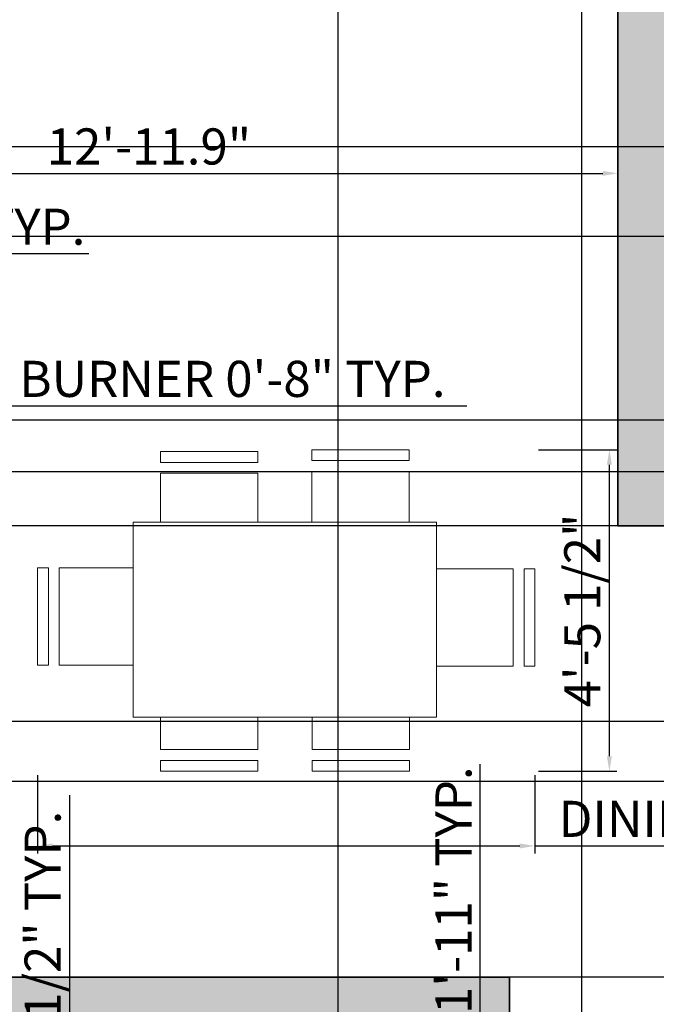
# Model space of a CAD drawing. Units: inches. Extents: x -40 to 424, y -33 to 568.
# Tile 5 of 8: x 66 to 171, y 275 to 438. Entities that reach past the tile are written whole.
import ezdxf

# ---------------------------------------------------------------- set-up
doc = ezdxf.new("R2010")
doc.units = ezdxf.units.IN
doc.linetypes.add('ACAD_ISO02W100', pattern=[15, 12, -3])
for name, color, linetype, lineweight in [('A-ANNO-DIMS', 7, 'Continuous', 18), ('A-FURN', 7, 'Continuous', 18), ('A-WALL-OVHD', 7, 'ACAD_ISO02W100', 18), ('A-WALL-PATT', 30, 'Continuous', 13), ('wall', 7, 'Continuous', 35)]:
    doc.layers.add(name, color=color, linetype=linetype, lineweight=lineweight)
doc.styles.get("Standard").update_dxf_attribs({"font": 'arial.ttf'})
doc.dimstyles.new('ISO-25', dxfattribs={"dimtxt": 6, "dimasz": 2.5, "dimexe": 1.25, "dimexo": 0.625, "dimtad": 1, "dimdec": 1, "dimlunit": 3, "dimtxsty": 'Standard', "dimcen": 2.5, "dimadec": 0, "dimazin": 0, "dimtfac": 1, "dimtdec": 1, "dimtmove": 0, "dimatfit": 3, "dimfxl": 1, "dimarcsym": 0})

# ---------------------------------------------------------------- blocks, each defined once
blk = doc.blocks.new('A$C6F2E0C66')
for p, q in [((0.5675, 1.4758), (0.5675, 1.4258)), ((1.0175, 1.4758), (0.5675, 1.4758)), ((1.0175, 1.4258), (1.0175, 1.4758)), ((1.2673, 1.4847), (1.2673, 1.4347)), ((1.7173, 1.4847), (1.2673, 1.4847)), ((1.7173, 1.4347), (1.7173, 1.4847)), ((0.5675, 1.4258), (1.0175, 1.4258)), ((1.2673, 1.4347), (1.7173, 1.4347)), ((0.5675, 1.3758), (0.5675, 1.15)), ((1.0175, 1.3758), (0.5675, 1.3758)), ((1.0175, 1.15), (1.0175, 1.3758)), ((1.2673, 1.3847), (1.2673, 1.15)), ((1.7173, 1.3847), (1.2673, 1.3847)), ((1.7173, 1.15), (1.7173, 1.3847)), ((0.4423, 1.15), (0.4423, 0.25)), ((1.8423, 1.15), (0.4423, 1.15)), ((1.8423, 0.25), (1.8423, 1.15)), ((0, 0.9395), (0, 0.4895)), ((0.05, 0.9395), (0, 0.9395)), ((0.05, 0.4895), (0.05, 0.9395)), ((0.4423, 0.9395), (0.1, 0.9395)), ((0.1, 0.9395), (0.1, 0.4895)), ((2.197, 0.9346), (1.8423, 0.9346)), ((2.197, 0.4846), (2.197, 0.9346)), ((2.247, 0.9346), (2.247, 0.4846)), ((2.297, 0.9346), (2.247, 0.9346)), ((2.297, 0.4846), (2.297, 0.9346)), ((0, 0.4895), (0.05, 0.4895)), ((0.1, 0.4895), (0.4423, 0.4895)), ((1.8423, 0.4846), (2.197, 0.4846)), ((2.247, 0.4846), (2.297, 0.4846)), ((0.4423, 0.25), (1.8423, 0.25)), ((0.5675, 0.25), (0.5675, 0.1)), ((1.0175, 0.1), (1.0175, 0.25)), ((1.2678, 0.25), (1.2678, 0.1)), ((1.7178, 0.1), (1.7178, 0.25)), ((0.5675, 0.1), (1.0175, 0.1)), ((1.2678, 0.1), (1.7178, 0.1)), ((0.5675, 0.05), (0.5675, 0)), ((1.0175, 0.05), (0.5675, 0.05)), ((1.0175, 0), (1.0175, 0.05)), ((1.2678, 0.05), (1.2678, 0)), ((1.7178, 0.05), (1.2678, 0.05)), ((1.7178, 0), (1.7178, 0.05)), ((0.5675, 0), (1.0175, 0)), ((1.2678, 0), (1.7178, 0))]:
    blk.add_line(p, q)
blk = doc.blocks.new('*D28')
at = {"layer": 'A-ANNO-DIMS', "color": 0, "lineweight": -2, "transparency": 16777216}
for p, q in [((9.08, 457.74), (9.08, 411.34)), ((165, 457.74), (165, 411.34)), ((11.58, 412.59), (162.5, 412.59))]:
    blk.add_line(p, q, dxfattribs=at)
at = {"layer": 'A-ANNO-DIMS', "color": 0, "transparency": 16777216}
for points in [[(11.58, 413.01), (11.58, 412.18), (9.08, 412.59)], [(162.5, 413.01), (162.5, 412.18), (165, 412.59)]]:
    blk.add_solid(points, dxfattribs=at)
at = {"layer": 'Defpoints', "color": 0, "transparency": 16777216}
for p in [(9.08, 458.36), (165, 458.36), (165, 412.59)]:
    blk.add_point(p, dxfattribs=at)
at = {"layer": 'A-ANNO-DIMS', "color": 0, "transparency": 16777216, "insert": (87.04, 416.28), "char_height": 6, "attachment_point": 5}
blk.add_mtext('12\'-11.9"', dxfattribs=at)
blk = doc.blocks.new('*D56')
at = {"layer": 'A-ANNO-DIMS', "color": 0, "lineweight": -2, "transparency": 16777216}
for p, q in [((142.1, 270), (142.1, 314.42)), ((134.16, 270), (143.35, 270)), ((142.1, 249.67), (142.1, 267.5)), ((134.16, 247.17), (143.35, 247.17))]:
    blk.add_line(p, q, dxfattribs=at)
at = {"layer": 'A-ANNO-DIMS', "color": 0, "transparency": 16777216}
for points in [[(141.68, 267.5), (142.51, 267.5), (142.1, 270)], [(141.68, 249.67), (142.51, 249.67), (142.1, 247.17)]]:
    blk.add_solid(points, dxfattribs=at)
at = {"layer": 'Defpoints', "color": 0, "transparency": 16777216}
for p in [(133.54, 270), (142.1, 270), (133.54, 247.17)]:
    blk.add_point(p, dxfattribs=at)
at = {"layer": 'A-ANNO-DIMS', "color": 0, "transparency": 16777216, "insert": (138.46, 293.46), "char_height": 6, "attachment_point": 5, "rotation": 90}
blk.add_mtext('1\'-11" TYP.', dxfattribs=at)
blk = doc.blocks.new('*D59')
at = {"layer": 'A-ANNO-DIMS', "color": 0, "lineweight": -2, "transparency": 16777216}
for p, q in [((73.87, 204.92), (73.87, 309.26)), ((83.22, 204.92), (72.62, 204.92)), ((73.87, 140.98), (73.87, 202.42)), ((83.22, 138.48), (72.62, 138.48))]:
    blk.add_line(p, q, dxfattribs=at)
at = {"layer": 'A-ANNO-DIMS', "color": 0, "transparency": 16777216}
for points in [[(73.46, 202.42), (74.29, 202.42), (73.87, 204.92)], [(73.46, 140.98), (74.29, 140.98), (73.87, 138.48)]]:
    blk.add_solid(points, dxfattribs=at)
at = {"layer": 'Defpoints', "color": 0, "transparency": 16777216}
for p in [(73.87, 204.92), (83.84, 204.92), (83.84, 138.48)]:
    blk.add_point(p, dxfattribs=at)
at = {"layer": 'A-ANNO-DIMS', "color": 0, "transparency": 16777216, "insert": (70.14, 258.34), "char_height": 6, "attachment_point": 5, "rotation": 90}
blk.add_mtext('LOW TABLE 5\'-6 1/2" TYP.', dxfattribs=at)
blk = doc.blocks.new('*D61')
at = {"layer": 'A-ANNO-DIMS', "color": 0, "lineweight": -2, "transparency": 16777216}
for p, q in [((68.52, 312.6), (68.52, 299.57)), ((151.21, 312.6), (151.21, 299.57)), ((71.02, 300.82), (148.71, 300.82)), ((151.21, 300.82), (239.55, 300.82))]:
    blk.add_line(p, q, dxfattribs=at)
at = {"layer": 'A-ANNO-DIMS', "color": 0, "transparency": 16777216}
for points in [[(71.02, 301.23), (71.02, 300.4), (68.52, 300.82)], [(148.71, 301.23), (148.71, 300.4), (151.21, 300.82)]]:
    blk.add_solid(points, dxfattribs=at)
at = {"layer": 'Defpoints', "color": 0, "transparency": 16777216}
for p in [(68.52, 313.22), (151.21, 313.22), (151.21, 300.82)]:
    blk.add_point(p, dxfattribs=at)
at = {"layer": 'A-ANNO-DIMS', "color": 0, "transparency": 16777216, "insert": (196.63, 304.54), "char_height": 6, "attachment_point": 5}
blk.add_mtext('DINING SET 6\'-10 1/2"', dxfattribs=at)
blk = doc.blocks.new('*D62')
at = {"layer": 'A-ANNO-DIMS', "color": 0, "lineweight": -2, "transparency": 16777216}
for p, q in [((151.83, 366.67), (164.86, 366.67)), ((163.61, 315.72), (163.61, 364.17)), ((151.83, 313.22), (164.86, 313.22))]:
    blk.add_line(p, q, dxfattribs=at)
at = {"layer": 'A-ANNO-DIMS', "color": 0, "transparency": 16777216}
for points in [[(163.2, 364.17), (164.03, 364.17), (163.61, 366.67)], [(163.2, 315.72), (164.03, 315.72), (163.61, 313.22)]]:
    blk.add_solid(points, dxfattribs=at)
at = {"layer": 'Defpoints', "color": 0, "transparency": 16777216}
for p in [(151.21, 366.67), (163.61, 366.67), (151.21, 313.22)]:
    blk.add_point(p, dxfattribs=at)
at = {"layer": 'A-ANNO-DIMS', "color": 0, "transparency": 16777216, "insert": (159.88, 339.94), "char_height": 6, "attachment_point": 5, "rotation": 90}
blk.add_mtext('4\'-5 1/2"', dxfattribs=at)
blk = doc.blocks.new('*D72')
at = {"layer": 'A-ANNO-DIMS', "color": 0, "lineweight": -2, "transparency": 16777216}
for p, q in [((31, 399.25), (28.5, 399.25)), ((33.5, 399.5), (33.5, 400.5)), ((33.5, 399.25), (34.25, 399.25)), ((34.25, 399.5), (34.25, 400.5)), ((36.75, 399.25), (77.07, 399.25))]:
    blk.add_line(p, q, dxfattribs=at)
at = {"layer": 'A-ANNO-DIMS', "color": 0, "transparency": 16777216}
for points in [[(31, 399.67), (31, 398.83), (33.5, 399.25)], [(36.75, 399.67), (36.75, 398.83), (34.25, 399.25)]]:
    blk.add_solid(points, dxfattribs=at)
at = {"layer": 'Defpoints', "color": 0, "transparency": 16777216}
for p in [(34.25, 399.25), (33.5, 398.88), (34.25, 398.88)]:
    blk.add_point(p, dxfattribs=at)
at = {"layer": 'A-ANNO-DIMS', "color": 0, "transparency": 16777216, "insert": (58.16, 402.94), "char_height": 6, "attachment_point": 5}
blk.add_mtext('0\'-1" TYP.', dxfattribs=at)
blk = doc.blocks.new('*D73')
at = {"layer": 'A-ANNO-DIMS', "color": 0, "lineweight": -2, "transparency": 16777216}
for p, q in [((23, 374.5), (23, 372.68)), ((25.5, 373.93), (28.5, 373.93)), ((31, 374.5), (31, 372.68)), ((31, 373.93), (139.9, 373.93))]:
    blk.add_line(p, q, dxfattribs=at)
at = {"layer": 'A-ANNO-DIMS', "color": 0, "transparency": 16777216}
for points in [[(25.5, 374.34), (25.5, 373.51), (23, 373.93)], [(28.5, 374.34), (28.5, 373.51), (31, 373.93)]]:
    blk.add_solid(points, dxfattribs=at)
at = {"layer": 'Defpoints', "color": 0, "transparency": 16777216}
for p in [(23, 375.13), (31, 375.13), (31, 373.93)]:
    blk.add_point(p, dxfattribs=at)
at = {"layer": 'A-ANNO-DIMS', "color": 0, "transparency": 16777216, "insert": (86.7, 377.66), "char_height": 6, "attachment_point": 5}
blk.add_mtext('FRONT BURNER 0\'-8" TYP.', dxfattribs=at)
blk = doc.blocks.new('*D89')
at = {"layer": 'A-ANNO-DIMS', "color": 0, "lineweight": -2, "transparency": 16777216}
for p, q in [((374.38, 417), (-28.55, 417)), ((-27.3, 365.5), (-27.3, 414.5)), ((374.38, 363), (-28.55, 363))]:
    blk.add_line(p, q, dxfattribs=at)
at = {"layer": 'A-ANNO-DIMS', "color": 0, "transparency": 16777216}
for points in [[(-27.72, 414.5), (-26.88, 414.5), (-27.3, 417)], [(-27.72, 365.5), (-26.88, 365.5), (-27.3, 363)]]:
    blk.add_solid(points, dxfattribs=at)
at = {"layer": 'Defpoints', "color": 0, "transparency": 16777216}
for p in [(-27.3, 417), (375, 417), (375, 363)]:
    blk.add_point(p, dxfattribs=at)
at = {"layer": 'A-ANNO-DIMS', "color": 0, "transparency": 16777216, "insert": (-30.99, 390), "char_height": 6, "attachment_point": 5, "rotation": 90}
blk.add_mtext('4\'-6"', dxfattribs=at)
blk = doc.blocks.new('*D92')
at = {"layer": 'A-ANNO-DIMS', "color": 0, "lineweight": -2, "transparency": 16777216}
for p, q in [((118.47, 470.38), (118.47, -28.55)), ((159, 470.38), (159, -28.55)), ((120.97, -27.3), (156.5, -27.3))]:
    blk.add_line(p, q, dxfattribs=at)
at = {"layer": 'A-ANNO-DIMS', "color": 0, "transparency": 16777216}
for points in [[(120.97, -26.88), (120.97, -27.72), (118.47, -27.3)], [(156.5, -26.88), (156.5, -27.72), (159, -27.3)]]:
    blk.add_solid(points, dxfattribs=at)
at = {"layer": 'Defpoints', "color": 0, "transparency": 16777216}
for p in [(118.47, 471), (159, 471), (159, -27.3)]:
    blk.add_point(p, dxfattribs=at)
at = {"layer": 'A-ANNO-DIMS', "color": 0, "transparency": 16777216, "insert": (138.73, -23.57), "char_height": 6, "attachment_point": 5}
blk.add_mtext('3\'-4 1/2"', dxfattribs=at)
blk = doc.blocks.new('*D97')
at = {"layer": 'A-ANNO-DIMS', "color": 0, "lineweight": -2, "transparency": 16777216}
for p, q in [((253.88, 311.5), (-28.55, 311.5)), ((-27.3, 281.5), (-27.3, 309)), ((253.88, 279), (-28.55, 279))]:
    blk.add_line(p, q, dxfattribs=at)
at = {"layer": 'A-ANNO-DIMS', "color": 0, "transparency": 16777216}
for points in [[(-27.72, 309), (-26.88, 309), (-27.3, 311.5)], [(-27.72, 281.5), (-26.88, 281.5), (-27.3, 279)]]:
    blk.add_solid(points, dxfattribs=at)
at = {"layer": 'Defpoints', "color": 0, "transparency": 16777216}
for p in [(-27.3, 311.5), (254.5, 311.5), (254.5, 279)]:
    blk.add_point(p, dxfattribs=at)
at = {"layer": 'A-ANNO-DIMS', "color": 0, "transparency": 16777216, "insert": (-31.03, 295.25), "char_height": 6, "attachment_point": 5, "rotation": 90}
blk.add_mtext('2\'-8 1/2"', dxfattribs=at)
blk = doc.blocks.new('*D99')
at = {"layer": 'A-ANNO-DIMS', "color": 0, "lineweight": -2, "transparency": 16777216}
for p, q in [((244.61, 354), (-28.55, 354)), ((-27.3, 324), (-27.3, 351.5)), ((244.61, 321.5), (-28.55, 321.5))]:
    blk.add_line(p, q, dxfattribs=at)
at = {"layer": 'A-ANNO-DIMS', "color": 0, "transparency": 16777216}
for points in [[(-27.72, 351.5), (-26.88, 351.5), (-27.3, 354)], [(-27.72, 324), (-26.88, 324), (-27.3, 321.5)]]:
    blk.add_solid(points, dxfattribs=at)
at = {"layer": 'Defpoints', "color": 0, "transparency": 16777216}
for p in [(-27.3, 354), (245.23, 354), (245.23, 321.5)]:
    blk.add_point(p, dxfattribs=at)
at = {"layer": 'A-ANNO-DIMS', "color": 0, "transparency": 16777216, "insert": (-31.03, 337.75), "char_height": 6, "attachment_point": 5, "rotation": 90}
blk.add_mtext('2\'-8 1/2"', dxfattribs=at)
blk = doc.blocks.new('*D103')
at = {"layer": 'A-ANNO-DIMS', "color": 0, "lineweight": -2, "transparency": 16777216}
for p, q in [((411.3, 402.13), (411.3, 435.91)), ((34.13, 402.13), (412.55, 402.13)), ((411.3, 374.13), (411.3, 399.63)), ((34.13, 371.63), (412.55, 371.63))]:
    blk.add_line(p, q, dxfattribs=at)
at = {"layer": 'A-ANNO-DIMS', "color": 0, "transparency": 16777216}
for points in [[(410.88, 399.63), (411.72, 399.63), (411.3, 402.13)], [(410.88, 374.13), (411.72, 374.13), (411.3, 371.63)]]:
    blk.add_solid(points, dxfattribs=at)
at = {"layer": 'Defpoints', "color": 0, "transparency": 16777216}
for p in [(33.5, 402.13), (411.3, 402.13), (33.5, 371.63)]:
    blk.add_point(p, dxfattribs=at)
at = {"layer": 'A-ANNO-DIMS', "color": 0, "transparency": 16777216, "insert": (407.57, 420.27), "char_height": 6, "attachment_point": 5, "rotation": 90}
blk.add_mtext('2\'-6 1/2"', dxfattribs=at)

msp = doc.modelspace()

# ---------------------------------------------------------------- hatches: boundary and pattern name
at = {"layer": 'A-WALL-PATT'}
h = msp.add_hatch(color=256, dxfattribs=at)
h.dxf.hatch_style = 1
h.paths.add_polyline_path([(9, 399), (0, 399), (0, 351), (9, 351)])
h.paths.add_polyline_path([(9, 303), (0, 303), (0, 210), (9, 210)])
h.paths.add_polyline_path([(9, 150), (0, 150), (0, 0), (384, 0), (384, 69), (375, 69), (375, 62.24), (375, 9), (9, 9)])
h.paths.add_polyline_path([(210, 177), (216, 177), (216, 186), (210, 186), (210, 216), (201, 216), (201, 90), (195, 90), (195, 81), (201, 81), (201, 9), (210, 9)])
h.paths.add_polyline_path([(384, 216), (375, 216), (375, 117), (384, 117)])
h.paths.add_polyline_path([(384, 298.5), (375, 298.5), (375, 279), (375, 240), (384, 240)])
h.paths.add_polyline_path([(384, 417), (375, 417), (375, 334.5), (384, 334.5)])
h.paths.add_polyline_path([(384, 528), (216, 528), (216, 519), (375, 519), (375, 465), (384, 465)])
h.paths.add_polyline_path([(192, 528), (0, 528), (0, 511.5), (9, 511.5), (9, 519), (192, 519)])
h.paths.add_polyline_path([(9, 487.5), (0, 487.5), (0, 447), (9, 447)])
h.paths.add_polyline_path([(111, 480), (9, 480), (9, 471), (111, 471)])
h.paths.add_polyline_path([(174, 519), (165, 519), (165, 354), (174, 354)])
h.paths.add_polyline_path([(243, 426), (237.86, 426), (234, 426), (234, 420), (174, 420), (174, 411), (234, 411), (234, 405), (239.14, 405), (243, 405)])
h.paths.add_polyline_path([(243, 519), (234, 519), (234, 460.14, -0.031638), (237.86, 460.2), (237.86, 462), (243, 462)])
h.paths.add_polyline_path([(243, 369), (234, 369), (234, 354), (375, 354), (375, 363), (243, 363)])
h.paths.add_polyline_path([(375, 279), (195, 279), (195, 270), (201, 270), (201, 264), (210, 264), (210, 270), (375, 270)])
h.paths.add_polyline_path([(291, 270), (282, 270), (282, 222), (286.29, 222), (291, 222)])
h.paths.add_polyline_path([(375, 186), (291, 186), (291, 192), (282, 192), (282, 186), (252, 186), (252, 180.86), (252, 177), (375, 177)])
h.paths.add_polyline_path([(147, 279), (9, 279), (9, 270), (147, 270)])

# ---------------------------------------------------------------- linework, layer by layer
at = {"layer": 'A-WALL-OVHD'}
msp.add_line((195, 279), (147, 279), dxfattribs=at)
at = {"layer": 'wall'}
for p, q in [((165, 519), (165, 354)), ((174, 354), (165, 354)), ((9, 279), (147, 279)), ((147, 279), (147, 270))]:
    msp.add_line(p, q, dxfattribs=at)

# ---------------------------------------------------------------- block references
at = {"layer": 'A-FURN', "xscale": 36, "yscale": 36, "zscale": 36}
msp.add_blockref('A$C6F2E0C66', (68.52, 313.22), dxfattribs=at)

# ---------------------------------------------------------------- dimensions: what is measured, and where the dimension line sits
at = {"layer": 'A-ANNO-DIMS'}
for base, p1, p2, override, picture, middle in [((159, -27.3), (118.47, 471), (159, 471), {"dimdec": 1, "dimlfac": 1, "dimrnd": 0, "dimzin": 1, "dimdsep": 46, "dimlunit": 4, "dimfrac": 2}, '*D92', (138.73, -23.57)), ((165, 412.59), (9.08, 458.36), (165, 458.36), {"dimclrd": 0, "dimclre": 0, "dimclrt": 0}, '*D28', (87.04, 416.28))]:
    dim = msp.add_linear_dim(base=base, p1=p1, p2=p2, dimstyle='ISO-25', override=override, dxfattribs=at)
    dim.commit()
    dim.dimension.update_dxf_attribs({"geometry": picture, "text_midpoint": middle})
for base, p1, p2, picture, middle in [((411.3, 402.13), (33.5, 371.63), (33.5, 402.13), '*D103', (407.57, 420.27)), ((-27.3, 417), (375, 363), (375, 417), '*D89', (-30.99, 390)), ((163.6119, 366.6685), (151.2081, 313.2208), (151.2081, 366.6685), '*D62', (159.8846, 339.9446)), ((-27.3, 354), (245.23, 321.5), (245.23, 354), '*D99', (-31.03, 337.75)), ((-27.3, 311.5), (254.5, 279), (254.5, 311.5), '*D97', (-31.03, 295.25))]:
    dim = msp.add_linear_dim(base=base, p1=p1, p2=p2, angle=90, dimstyle='ISO-25', override={"dimdec": 1, "dimlfac": 1, "dimrnd": 0, "dimzin": 1, "dimdsep": 46, "dimlunit": 4, "dimfrac": 2}, dxfattribs=at)
    dim.commit()
    dim.dimension.update_dxf_attribs({"geometry": picture, "text_midpoint": middle})
for base, p1, p2, text, picture, middle in [((34.25, 399.25069249), (33.5, 398.87569249), (34.25, 398.87569249), '<> TYP.', '*D72', (58.16149386, 402.93913042)), ((31, 373.93), (23, 375.13), (31, 375.13), 'FRONT BURNER <> TYP.', '*D73', (86.7, 377.66)), ((151.21, 300.82), (68.52, 313.22), (151.21, 313.22), 'DINING SET <>', '*D61', (196.63, 304.54))]:
    dim = msp.add_linear_dim(base=base, p1=p1, p2=p2, text=text, dimstyle='ISO-25', override={"dimdec": 1, "dimlfac": 1, "dimrnd": 0, "dimzin": 1, "dimdsep": 46, "dimlunit": 4, "dimfrac": 2}, dxfattribs=at)
    dim.commit()
    dim.dimension.update_dxf_attribs({"geometry": picture, "text_midpoint": middle})
for base, p1, p2, text, picture, middle in [((142.1, 270), (133.54, 247.17), (133.54, 270), '<> TYP.', '*D56', (138.46, 293.46)), ((73.87, 204.92), (83.84, 138.48), (83.84, 204.92), 'LOW TABLE <> TYP.', '*D59', (70.14, 258.34))]:
    dim = msp.add_linear_dim(base=base, p1=p1, p2=p2, angle=90, text=text, dimstyle='ISO-25', override={"dimdec": 1, "dimlfac": 1, "dimrnd": 0, "dimzin": 1, "dimdsep": 46, "dimlunit": 4, "dimfrac": 2}, dxfattribs=at)
    dim.commit()
    dim.dimension.update_dxf_attribs({"geometry": picture, "text_midpoint": middle})

doc.saveas('drawing.dxf')
